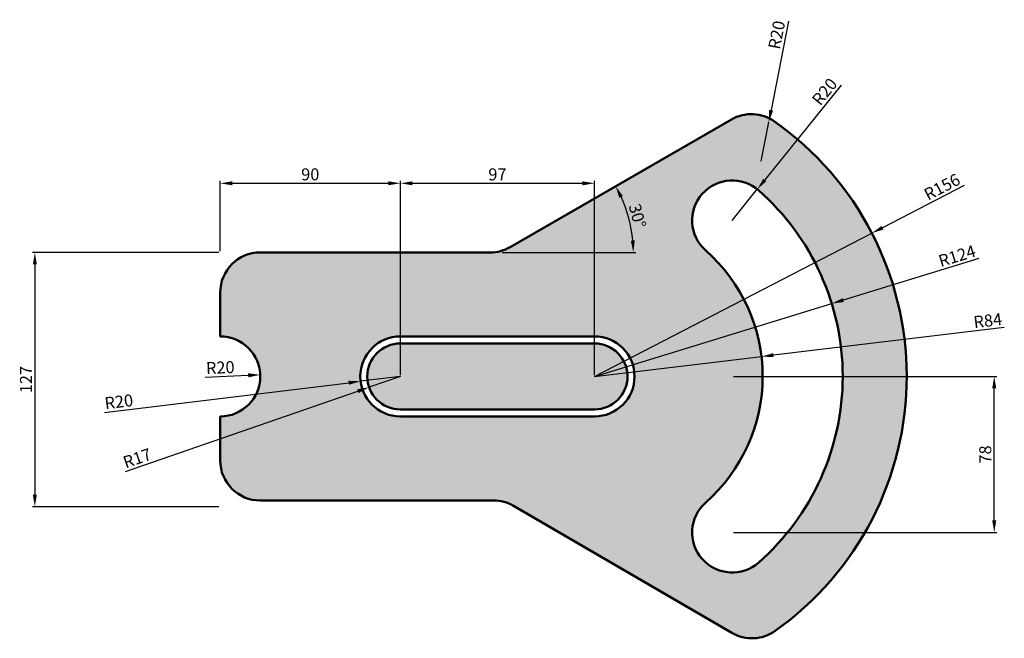
# Model space of a CAD drawing. Units: millimetres. Extents: x 2036 to 2528, y 117 to 427.
import ezdxf

# ---------------------------------------------------------------- set-up
doc = ezdxf.new("R2010")
doc.units = ezdxf.units.MM
for name, color, linetype, lineweight in [('M-DIMS', 2, 'Continuous', 25), ('M-HATC', 8, 'Continuous', 18), ('M-OUTL', 7, 'Continuous', 50)]:
    doc.layers.add(name, color=color, linetype=linetype, lineweight=lineweight)
doc.styles.get("Standard").update_dxf_attribs({"font": 'arial.ttf'})
doc.dimstyles.new('ISO-25', dxfattribs={"dimtxt": 6, "dimasz": 6, "dimexe": 1.25, "dimexo": 0.625, "dimtad": 1, "dimdec": 0, "dimtxsty": 'Standard', "dimcen": 2.5, "dimadec": 0, "dimazin": 0, "dimtfac": 1, "dimtdec": 0, "dimtmove": 0, "dimatfit": 3, "dimfxl": 1, "dimarcsym": 0})

# ---------------------------------------------------------------- blocks, each defined once
blk = doc.blocks.new('*D1')
at = {"layer": 'Defpoints', "color": 0, "transparency": 16777216}
for p in [(2136.66, 248.21), (2156.64, 249.02)]:
    blk.add_point(p, dxfattribs=at)
at = {"layer": 'M-DIMS', "color": 0, "lineweight": -2, "transparency": 16777216}
blk.add_line((2129.1, 247.9), (2150.65, 248.78), dxfattribs=at)
at = {"layer": 'M-DIMS', "color": 0, "transparency": 16777216}
blk.add_solid([(2150.61, 249.78), (2150.69, 247.78), (2156.64, 249.02)], dxfattribs=at)
at = {"layer": 'M-DIMS', "color": 0, "transparency": 16777216, "insert": (2136.73, 251.9), "char_height": 6, "attachment_point": 5, "rotation": 2.3313}
blk.add_mtext('R20', dxfattribs=at)
blk = doc.blocks.new('*D2')
at = {"layer": 'Defpoints', "color": 0, "transparency": 16777216}
for p in [(2226.66, 248.21), (2211.07, 242.81)]:
    blk.add_point(p, dxfattribs=at)
at = {"layer": 'M-DIMS', "color": 0, "lineweight": -2, "transparency": 16777216}
for p, q in [((2226.66, 248.21), (2211.07, 242.81)), ((2089.27, 200.63), (2205.4, 240.84))]:
    blk.add_line(p, q, dxfattribs=at)
at = {"layer": 'M-DIMS', "color": 0, "transparency": 16777216}
blk.add_solid([(2205.07, 241.79), (2205.72, 239.9), (2211.07, 242.81)], dxfattribs=at)
at = {"layer": 'M-DIMS', "color": 0, "transparency": 16777216, "insert": (2095.45, 206.62), "char_height": 6, "attachment_point": 5, "rotation": 19.099}
blk.add_mtext('R17', dxfattribs=at)
blk = doc.blocks.new('*D3')
at = {"layer": 'Defpoints', "color": 0, "transparency": 16777216}
for p in [(2226.66, 248.21), (2206.81, 245.79)]:
    blk.add_point(p, dxfattribs=at)
at = {"layer": 'M-DIMS', "color": 0, "lineweight": -2, "transparency": 16777216}
for p, q in [((2226.66, 248.21), (2206.81, 245.79)), ((2078.83, 230.23), (2200.85, 245.07))]:
    blk.add_line(p, q, dxfattribs=at)
at = {"layer": 'M-DIMS', "color": 0, "transparency": 16777216}
blk.add_solid([(2200.73, 246.06), (2200.97, 244.07), (2206.81, 245.79)], dxfattribs=at)
at = {"layer": 'M-DIMS', "color": 0, "transparency": 16777216, "insert": (2086.11, 234.83), "char_height": 6, "attachment_point": 5, "rotation": 6.9344}
blk.add_mtext('R20', dxfattribs=at)
blk = doc.blocks.new('*D4')
at = {"layer": 'Defpoints', "color": 0, "transparency": 16777216}
for p in [(2323.66, 344.77), (2226.66, 248.21), (2323.66, 248.21)]:
    blk.add_point(p, dxfattribs=at)
at = {"layer": 'M-DIMS', "color": 0, "lineweight": -2, "transparency": 16777216}
for p, q in [((2226.66, 248.83), (2226.66, 346.02)), ((2232.66, 344.77), (2317.66, 344.77)), ((2323.66, 248.83), (2323.66, 346.02))]:
    blk.add_line(p, q, dxfattribs=at)
at = {"layer": 'M-DIMS', "color": 0, "transparency": 16777216}
for points in [[(2232.66, 345.77), (2232.66, 343.77), (2226.66, 344.77)], [(2317.66, 345.77), (2317.66, 343.77), (2323.66, 344.77)]]:
    blk.add_solid(points, dxfattribs=at)
at = {"layer": 'M-DIMS', "color": 0, "transparency": 16777216, "insert": (2275.16, 348.46), "char_height": 6, "attachment_point": 5}
blk.add_mtext('97', dxfattribs=at)
blk = doc.blocks.new('*D5')
at = {"layer": 'Defpoints', "color": 0, "transparency": 16777216}
for p in [(2462.24, 319.84), (2323.66, 248.21)]:
    blk.add_point(p, dxfattribs=at)
at = {"layer": 'M-DIMS', "color": 0, "lineweight": -2, "transparency": 16777216}
for p, q in [((2508.33, 343.66), (2467.57, 322.59)), ((2323.66, 248.21), (2462.24, 319.84))]:
    blk.add_line(p, q, dxfattribs=at)
at = {"layer": 'M-DIMS', "color": 0, "transparency": 16777216}
blk.add_solid([(2467.11, 323.48), (2468.03, 321.7), (2462.24, 319.84)], dxfattribs=at)
at = {"layer": 'M-DIMS', "color": 0, "transparency": 16777216, "insert": (2497.64, 342.29), "char_height": 6, "attachment_point": 5, "rotation": 27.3335}
blk.add_mtext('R156', dxfattribs=at)
blk = doc.blocks.new('*D6')
at = {"layer": 'Defpoints', "color": 0, "transparency": 16777216}
for p in [(2442.19, 284.61), (2323.66, 248.21)]:
    blk.add_point(p, dxfattribs=at)
at = {"layer": 'M-DIMS', "color": 0, "lineweight": -2, "transparency": 16777216}
for p, q in [((2515.74, 307.21), (2447.93, 286.38)), ((2323.66, 248.21), (2442.19, 284.61))]:
    blk.add_line(p, q, dxfattribs=at)
at = {"layer": 'M-DIMS', "color": 0, "transparency": 16777216}
blk.add_solid([(2447.64, 287.33), (2448.22, 285.42), (2442.19, 284.61)], dxfattribs=at)
at = {"layer": 'M-DIMS', "color": 0, "transparency": 16777216, "insert": (2505.01, 307.71), "char_height": 6, "attachment_point": 5, "rotation": 17.0746}
blk.add_mtext('R124', dxfattribs=at)
blk = doc.blocks.new('*D7')
at = {"layer": 'Defpoints', "color": 0, "transparency": 16777216}
for p in [(2407.07, 258.16), (2323.66, 248.21)]:
    blk.add_point(p, dxfattribs=at)
at = {"layer": 'M-DIMS', "color": 0, "lineweight": -2, "transparency": 16777216}
for p, q in [((2528.4, 272.63), (2413.03, 258.87)), ((2323.66, 248.21), (2407.07, 258.16))]:
    blk.add_line(p, q, dxfattribs=at)
at = {"layer": 'M-DIMS', "color": 0, "transparency": 16777216}
blk.add_solid([(2412.91, 259.86), (2413.14, 257.87), (2407.07, 258.16)], dxfattribs=at)
at = {"layer": 'M-DIMS', "color": 0, "transparency": 16777216, "insert": (2520.23, 275.37), "char_height": 6, "attachment_point": 5, "rotation": 6.8018}
blk.add_mtext('R84', dxfattribs=at)
blk = doc.blocks.new('*D8')
at = {"layer": 'Defpoints', "color": 0, "transparency": 16777216}
for p in [(2405, 341.78), (2392.45, 326.21)]:
    blk.add_point(p, dxfattribs=at)
at = {"layer": 'M-DIMS', "color": 0, "lineweight": -2, "transparency": 16777216}
for p, q in [((2446.96, 393.87), (2408.76, 346.45)), ((2392.45, 326.21), (2405, 341.78))]:
    blk.add_line(p, q, dxfattribs=at)
at = {"layer": 'M-DIMS', "color": 0, "transparency": 16777216}
blk.add_solid([(2407.98, 347.08), (2409.54, 345.83), (2405, 341.78)], dxfattribs=at)
at = {"layer": 'M-DIMS', "color": 0, "transparency": 16777216, "insert": (2439.21, 390.12), "char_height": 6, "attachment_point": 5, "rotation": 51.1436}
blk.add_mtext('R20', dxfattribs=at)
blk = doc.blocks.new('*D9')
at = {"layer": 'Defpoints', "color": 0, "transparency": 16777216}
for p in [(2410.73, 375.39), (2406.9, 355.76)]:
    blk.add_point(p, dxfattribs=at)
at = {"layer": 'M-DIMS', "color": 0, "lineweight": -2, "transparency": 16777216}
for p, q in [((2420.55, 425.74), (2411.88, 381.28)), ((2406.9, 355.76), (2410.73, 375.39))]:
    blk.add_line(p, q, dxfattribs=at)
at = {"layer": 'M-DIMS', "color": 0, "transparency": 16777216}
blk.add_solid([(2410.89, 381.47), (2412.86, 381.09), (2410.73, 375.39)], dxfattribs=at)
at = {"layer": 'M-DIMS', "color": 0, "transparency": 16777216, "insert": (2415.44, 418.8), "char_height": 6, "attachment_point": 5, "rotation": 78.9572}
blk.add_mtext('R20', dxfattribs=at)
blk = doc.blocks.new('*D10')
at = {"layer": 'Defpoints', "color": 0, "transparency": 16777216}
for p in [(2136.66, 310.21), (2044.06, 183.09), (2136.66, 183.09)]:
    blk.add_point(p, dxfattribs=at)
at = {"layer": 'M-DIMS', "color": 0, "lineweight": -2, "transparency": 16777216}
for p, q in [((2136.03, 310.21), (2042.81, 310.21)), ((2044.06, 304.21), (2044.06, 189.09)), ((2136.03, 183.09), (2042.81, 183.09))]:
    blk.add_line(p, q, dxfattribs=at)
at = {"layer": 'M-DIMS', "color": 0, "transparency": 16777216}
for points in [[(2043.06, 304.21), (2045.06, 304.21), (2044.06, 310.21)], [(2043.06, 189.09), (2045.06, 189.09), (2044.06, 183.09)]]:
    blk.add_solid(points, dxfattribs=at)
at = {"layer": 'M-DIMS', "color": 0, "transparency": 16777216, "insert": (2040.43, 246.65), "char_height": 6, "attachment_point": 5, "rotation": 90}
blk.add_mtext('127', dxfattribs=at)
blk = doc.blocks.new('*D11')
at = {"layer": 'Defpoints', "color": 0, "transparency": 16777216}
for p in [(2226.66, 344.77), (2136.66, 310.21), (2226.66, 310.21)]:
    blk.add_point(p, dxfattribs=at)
at = {"layer": 'M-DIMS', "color": 0, "lineweight": -2, "transparency": 16777216}
for p, q in [((2136.66, 310.83), (2136.66, 346.02)), ((2142.66, 344.77), (2220.66, 344.77)), ((2226.66, 310.83), (2226.66, 346.02))]:
    blk.add_line(p, q, dxfattribs=at)
at = {"layer": 'M-DIMS', "color": 0, "transparency": 16777216}
for points in [[(2142.66, 345.77), (2142.66, 343.77), (2136.66, 344.77)], [(2220.66, 345.77), (2220.66, 343.77), (2226.66, 344.77)]]:
    blk.add_solid(points, dxfattribs=at)
at = {"layer": 'M-DIMS', "color": 0, "transparency": 16777216, "insert": (2181.66, 348.46), "char_height": 6, "attachment_point": 5}
blk.add_mtext('90', dxfattribs=at)
blk = doc.blocks.new('*D12')
at = {"layer": 'Defpoints', "color": 0, "transparency": 16777216}
for p in [(2392.04, 376.67), (2342.06, 321.69), (2156.66, 310.21), (2271.57, 310.21), (2281.57, 312.89)]:
    blk.add_point(p, dxfattribs=at)
at = {"layer": 'M-DIMS', "color": 0, "lineweight": -2, "transparency": 16777216}
blk.add_line((2277.55, 310.21), (2344.31, 310.21), dxfattribs=at)
blk.add_arc((2276.92, 310.21), 66.14, 5.1998, 24.8002, dxfattribs=at)
at = {"layer": 'M-DIMS', "color": 0, "transparency": 16777216}
for points in [[(2336.07, 337.49), (2337.85, 338.41), (2334.2, 343.27)], [(2343.79, 316.25), (2341.79, 316.15), (2343.06, 310.21)]]:
    blk.add_solid(points, dxfattribs=at)
at = {"layer": 'M-DIMS', "color": 0, "transparency": 16777216, "insert": (2344.37, 328.28), "char_height": 6, "attachment_point": 5, "rotation": 285}
blk.add_mtext('30°', dxfattribs=at)
blk = doc.blocks.new('*D13')
at = {"layer": 'Defpoints', "color": 0, "transparency": 16777216}
for p in [(2392.45, 248.21), (2523.36, 248.21), (2392.45, 170.21)]:
    blk.add_point(p, dxfattribs=at)
at = {"layer": 'M-DIMS', "color": 0, "lineweight": -2, "transparency": 16777216}
for p, q in [((2393.07, 248.21), (2524.61, 248.21)), ((2523.36, 176.21), (2523.36, 242.21)), ((2393.07, 170.21), (2524.61, 170.21))]:
    blk.add_line(p, q, dxfattribs=at)
at = {"layer": 'M-DIMS', "color": 0, "transparency": 16777216}
for points in [[(2522.36, 242.21), (2524.36, 242.21), (2523.36, 248.21)], [(2522.36, 176.21), (2524.36, 176.21), (2523.36, 170.21)]]:
    blk.add_solid(points, dxfattribs=at)
at = {"layer": 'M-DIMS', "color": 0, "transparency": 16777216, "insert": (2519.67, 209.21), "char_height": 6, "attachment_point": 5, "rotation": 90}
blk.add_mtext('78', dxfattribs=at)

msp = doc.modelspace()

# ---------------------------------------------------------------- hatches: boundary and pattern name
at = {"layer": 'M-HATC'}
h = msp.add_hatch(color=256, dxfattribs=at)
h.dxf.hatch_style = 1
h.set_gradient(color1=(0, 0, 255), color2=(255, 255, 0), tint=1)
h.paths.add_polyline_path([(2413.57, 375.69, 0.292387), (2392.04, 376.67), (2281.57, 312.89, -0.131652), (2271.57, 310.21), (2156.66, 310.21, 0.414214), (2136.66, 290.21), (2136.66, 268.21, -1), (2136.66, 228.21), (2136.66, 206.21, 0.414214), (2156.66, 186.21), (2273.15, 186.21, -0.132491), (2283.21, 183.49), (2392.32, 120.02, 0.294111), (2413.96, 121, 0.517461)])
h.paths.add_polyline_path([(2226.66, 268.21), (2323.66, 268.21, -1), (2323.66, 228.21), (2226.66, 228.21, -1)], flags=16)
h.paths.add_polyline_path([(2226.66, 264.71), (2323.66, 264.71, -1), (2323.66, 231.71), (2226.66, 231.71, -1)], flags=0)
h.paths.add_polyline_path([(2405.68, 341.21, -0.451416), (2405.68, 155.21, -1), (2379.22, 185.21, 0.451416), (2379.22, 311.21, -1)], flags=16)
h.paths.add_polyline_path([(2336.35, 334.14), (2340.4, 319), (2352.35, 322.2), (2348.29, 337.34)], flags=24)
h = msp.add_hatch(color=256, dxfattribs=at)
h.dxf.hatch_style = 1
h.paths.add_polyline_path([(2323.66, 264.71), (2226.66, 264.71, 1), (2226.66, 231.71), (2323.66, 231.71, 1)])

# ---------------------------------------------------------------- linework, layer by layer
at = {"layer": 'M-OUTL'}
for p, q in [((2281.57, 312.89), (2392.04, 376.67)), ((2156.66, 310.21), (2226.66, 310.21)), ((2156.66, 310.21), (2271.57, 310.21)), ((2136.66, 268.21), (2136.66, 290.21)), ((2226.66, 268.21), (2323.66, 268.21)), ((2226.66, 264.71), (2323.66, 264.71)), ((2226.66, 231.71), (2323.66, 231.71)), ((2136.66, 206.21), (2136.66, 228.21)), ((2226.66, 228.21), (2323.66, 228.21)), ((2156.66, 186.21), (2273.15, 186.21)), ((2283.21, 183.49), (2392.32, 120.02))]:
    msp.add_line(p, q, dxfattribs=at)
for centre, radius, start, end in [((2402.04, 359.35), 20, 54.8071, 120), ((2323.66, 248.21), 156, 305.3679, 54.8071), ((2392.45, 326.21), 20, 48.5904, 228.5904), ((2323.66, 248.21), 124, 311.4096, 48.5904), ((2156.66, 290.21), 20, 90, 180), ((2271.57, 330.21), 20, 270, 300), ((2323.66, 248.21), 84, 311.4096, 48.5904), ((2136.66, 248.21), 20, 270, 90), ((2226.66, 248.21), 20, 90, 270), ((2323.66, 248.21), 20, 270, 90), ((2226.66, 248.21), 16.5, 90, 270), ((2323.66, 248.21), 16.5, 270, 90), ((2156.66, 206.21), 20, 180, 270), ((2273.15, 166.21), 20, 59.8111, 90), ((2392.45, 170.21), 20, 131.4096, 311.4096), ((2402.38, 137.3), 20, 239.8111, 305.3679)]:
    msp.add_arc(centre, radius, start, end, dxfattribs=at)

# ---------------------------------------------------------------- dimensions: what is measured, and where the dimension line sits
at = {"layer": 'M-DIMS'}
for center, mpoint, picture, middle in [((2406.9, 355.76), (2410.73, 375.39), '*D9', (2419.06, 418.1)), ((2392.45, 326.21), (2405, 341.78), '*D8', (2442.08, 387.81)), ((2323.66, 248.21), (2462.24, 319.84), '*D5', (2499.34, 339.01)), ((2323.66, 248.21), (2442.19, 284.61), '*D6', (2506.07, 304.24)), ((2323.66, 248.21), (2407.07, 258.16), '*D7', (2520.67, 271.71)), ((2136.66, 248.21), (2156.64, 249.02), '*D1', (2136.88, 248.22)), ((2226.66, 248.21), (2206.81, 245.79), '*D3', (2086.55, 231.17)), ((2226.66, 248.21), (2211.07, 242.81), '*D2', (2096.64, 203.18))]:
    dim = msp.add_radius_dim(center=center, mpoint=mpoint, dimstyle='ISO-25', override={"dimclrd": 0, "dimclre": 0, "dimclrt": 0}, dxfattribs=at)
    dim.commit()
    dim.dimension.update_dxf_attribs({"geometry": picture, "text_midpoint": middle, "dimtype": 164})
dim = msp.add_angular_dim_2l(base=(2342.06, 321.69), line1=((2281.57, 312.89), (2392.04, 376.67)), line2=((2156.66, 310.21), (2271.57, 310.21)), dimstyle='ISO-25', override={"dimclrd": 0, "dimclre": 0, "dimclrt": 0}, dxfattribs=at)
dim.commit()
dim.dimension.update_dxf_attribs({"geometry": '*D12', "text_midpoint": (2344.37, 328.28)})
for base, p1, p2, picture, middle in [((2226.66, 344.77), (2136.66, 310.21), (2226.66, 310.21), '*D11', (2181.66, 348.46)), ((2323.66, 344.77), (2226.66, 248.21), (2323.66, 248.21), '*D4', (2275.16, 348.46))]:
    dim = msp.add_linear_dim(base=base, p1=p1, p2=p2, dimstyle='ISO-25', override={"dimclrd": 0, "dimclre": 0, "dimclrt": 0}, dxfattribs=at)
    dim.commit()
    dim.dimension.update_dxf_attribs({"geometry": picture, "text_midpoint": middle})
for base, p1, p2, picture, middle in [((2044.06, 183.09), (2136.66, 310.21), (2136.66, 183.09), '*D10', (2040.43, 246.65)), ((2523.36, 248.21), (2392.45, 170.21), (2392.45, 248.21), '*D13', (2519.67, 209.21))]:
    dim = msp.add_linear_dim(base=base, p1=p1, p2=p2, angle=90, dimstyle='ISO-25', override={"dimclrd": 0, "dimclre": 0, "dimclrt": 0}, dxfattribs=at)
    dim.commit()
    dim.dimension.update_dxf_attribs({"geometry": picture, "text_midpoint": middle})

doc.saveas('drawing.dxf')
